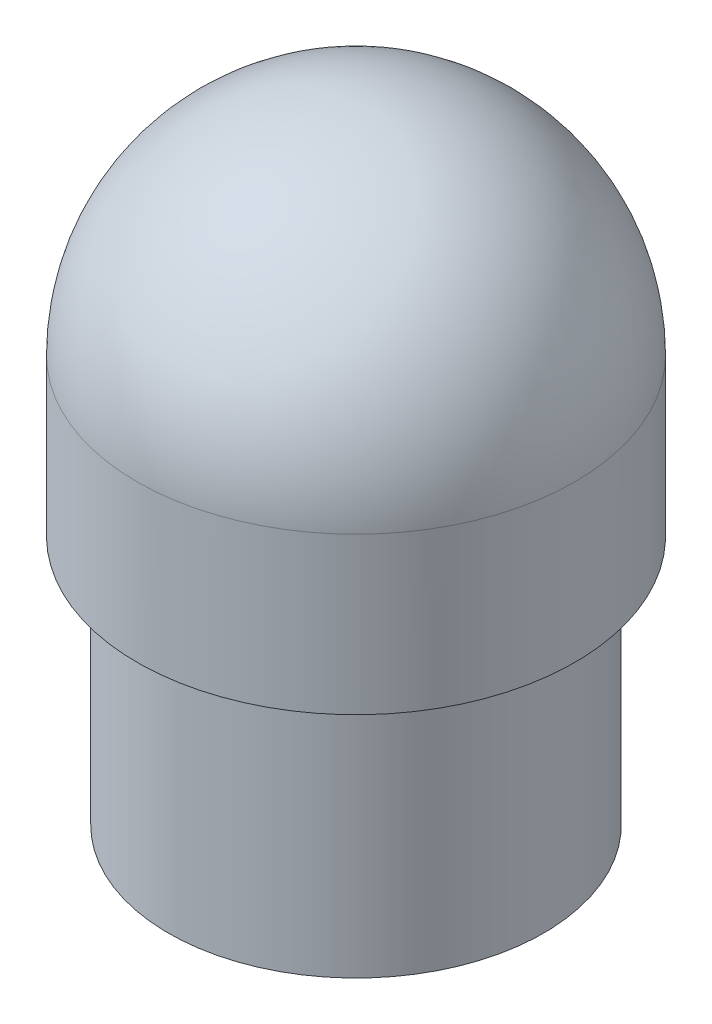
SolidWorks part; units mm, degrees
material "Plain Carbon Steel"
ref_plane "Front Plane" through (0, 0, 0) normal (0, 0, 1) x (1, 0, 0)
ref_plane "Top Plane" through (0, 0, 0) normal (0, 1, 0) x (1, 0, 0)
ref_plane "Right Plane" through (0, 0, 0) normal (1, 0, 0) x (0, 0, -1)
sketch "Pin Profile Sketch" plane through (0, 0, 0) normal (0, 0, 1) x (1, 0, 0)
  line L0 (0, 0) -> (15, 0)
  line L1 (15, 0) -> (15, 20)
  line L2 (15, 20) -> (17.5, 20)
  line L3 (17.5, 20) -> (17.5, 32.5)
  line L4 (0, 50) -> (0, 0)
  arc A0 (17.5, 32.5) -> (0, 50) centre (0, 32.5) ccw
  dimension "D1" = 17.5
  dimension "D2" = 50
  dimension "D3" = 20
  dimension "D4" = 15
  dimension "D5" = 17.5
revolve "Pin Body Revolve" add sketch "Pin Profile Sketch" angle 360 about L4
